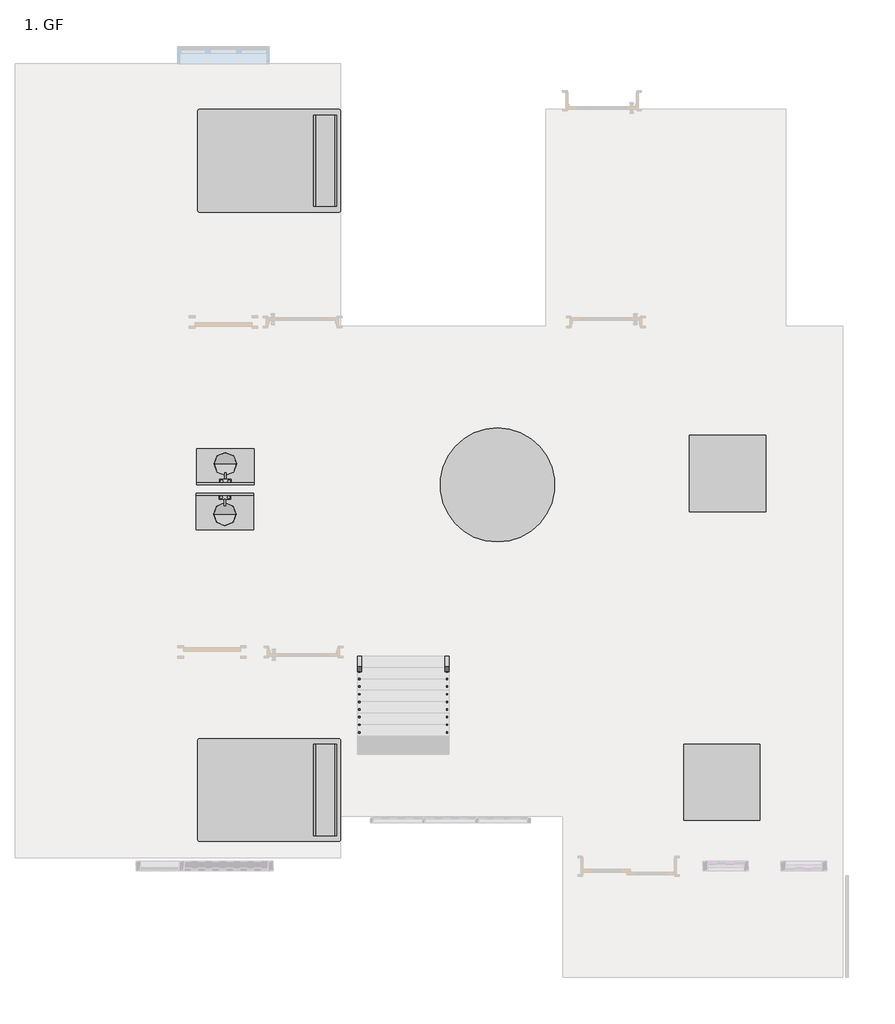
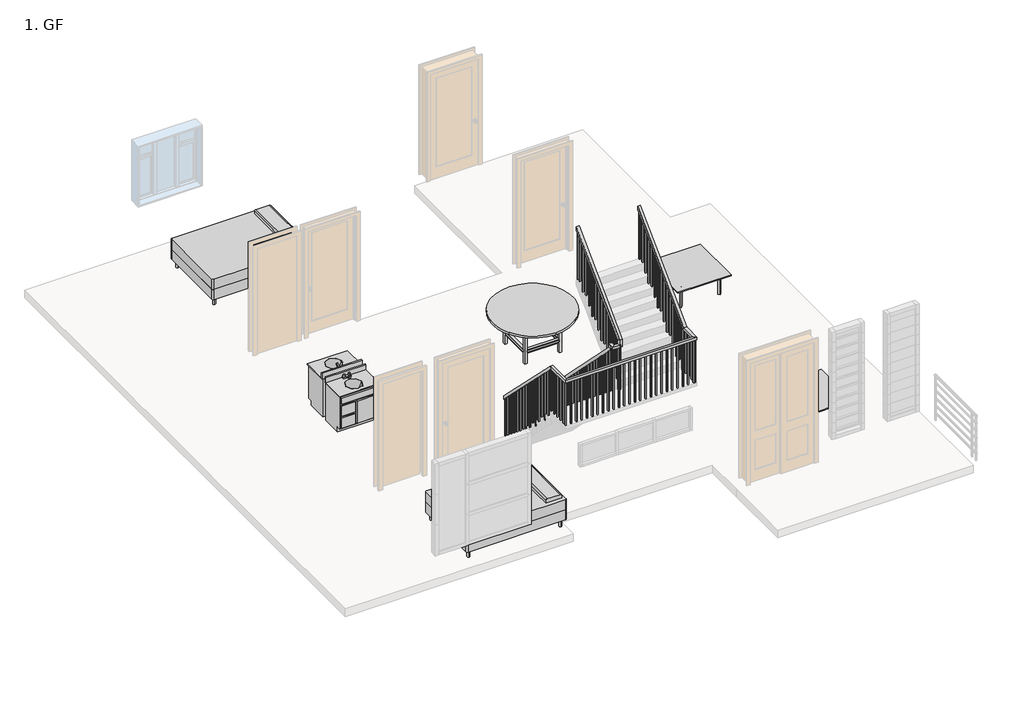
# One storey, part 3 of 3: 5 furniture elements, 2 flow terminals, 2 railings.
"""IFC4 building model written with IfcOpenShell, lengths in millimetres."""

from ifc_helpers import new_model, si_unit, frame, origin, place, context, project, spatial, polyline, outline, extrude, faceted_brep, transform, mapped, element, save
from components import flow_terminal_15267b2a, furniture_7b9c1204, furniture_52ef1662, furniture_86cdcdde

model = new_model("IFC4")

# Units and contexts
model_context = context("Model", 3, world=origin())
ifc_project = project(units=[si_unit("LENGTHUNIT", "METRE", prefix="MILLI")], contexts=[model_context])

# Site, building, storey
site = spatial("IfcSite", under=ifc_project)
building = spatial("IfcBuilding", under=site)
storey = spatial("IfcBuildingStorey", under=building, Name="1. GF", Elevation=609.6)

# Flow terminals
placement = place(None, origin())
flow_terminal_shape = flow_terminal_15267b2a(model_context)
element("IfcFlowTerminal", 1, ObjectType="Lavatory - Vanity : 30\"x18\" - Private", at=placement, inside=storey, context=model_context, shape_type="MappedRepresentation", body=[
    mapped(flow_terminal_shape, transform((-4529.7749552, 4478.4722789, 609.6), x_axis=(0.0, 1.0, 0.0), y_axis=(-1.0, 0.0, 0.0), z_axis=(0.0, 0.0, 1.0))),
])
element("IfcFlowTerminal", 2, ObjectType="Lavatory - Vanity : 30\"x18\" - Private", at=placement, inside=storey, context=model_context, shape_type="MappedRepresentation", body=[
    mapped(flow_terminal_shape, transform((-4536.1249552, 4365.7597789, 609.6), x_axis=(0.0, -1.0, 0.0), y_axis=(1.0, 0.0, 0.0), z_axis=(0.0, 0.0, 1.0))),
])

# Furniture
furniture_shape = furniture_7b9c1204(model_context)
element("IfcFurniture", 3, ObjectType="40\" x 40\"", at=placement, inside=storey, context=model_context, shape_type="MappedRepresentation", body=[
    mapped(furniture_shape, transform((2231.2053727, 4691.6266846, 609.6), x_axis=(1.0, 0.0, 0.0), y_axis=(0.0, 1.0, 0.0), z_axis=(0.0, 0.0, 1.0))),
])
element("IfcFurniture", 4, ObjectType="40\" x 40\"", at=placement, inside=storey, context=model_context, shape_type="MappedRepresentation", body=[
    mapped(furniture_shape, transform((2155.0053727, 570.4766846, 609.6), x_axis=(1.0, 0.0, 0.0), y_axis=(0.0, 1.0, 0.0), z_axis=(0.0, 0.0, 1.0))),
])
furniture_2_shape = furniture_52ef1662(model_context)
element("IfcFurniture", 5, ObjectType="Bed-Standard : Double 54\" x 75\"", at=placement, inside=storey, context=model_context, shape_type="MappedRepresentation", body=[
    mapped(furniture_2_shape, transform((-3899.9798732, 9075.1045534, 609.6), x_axis=(0.0, -1.0, 0.0), y_axis=(1.0, 0.0, 0.0), z_axis=(0.0, 0.0, 1.0))),
])
element("IfcFurniture", 6, ObjectType="Bed-Standard : Double 54\" x 75\"", at=placement, inside=storey, context=model_context, shape_type="MappedRepresentation", body=[
    mapped(furniture_2_shape, transform((-3899.9798732, 680.4045534, 609.6), x_axis=(0.0, -1.0, 0.0), y_axis=(1.0, 0.0, 0.0), z_axis=(0.0, 0.0, 1.0))),
])
furniture_3_shape = furniture_86cdcdde(model_context)
element("IfcFurniture", 7, ObjectType="Table-Dining Round w Chairs : 60\" Diameter", at=placement, inside=storey, context=model_context, shape_type="MappedRepresentation", body=[
    mapped(furniture_3_shape, transform((-1001.2569224, 4664.1447174, 609.6), x_axis=(1.0, 0.0, 0.0), y_axis=(0.0, 1.0, 0.0), z_axis=(0.0, 0.0, 1.0))),
])

# Railings
element("IfcRailing", 8, ObjectType="Handrail - Rectangular", at=placement, inside=storey, context=model_context, shape_type="SolidModel", body=[
    faceted_brep([(-2713.6749552, 2193.2660289, 1676.4), (-2713.6749552, 2193.2660289, 1604.557951), (-2764.4749552, 2193.2660289, 1604.557951), (-2764.4749552, 2193.2660289, 1676.4), (-2713.6749552, 669.2660289, 3200.4), (-2713.6749552, 648.2239799, 3149.6), (-2764.4749552, 648.2239799, 3149.6), (-2764.4749552, 669.2660289, 3200.4), (-2713.6749552, 224.7660289, 3200.4), (-2713.6749552, 224.7660289, 3149.6), (-2764.4749552, 173.9660289, 3149.6), (-2764.4749552, 173.9660289, 3200.4), (-300.6749552, 224.7660289, 3200.4), (-300.6749552, 224.7660289, 3149.6), (-249.8749552, 173.9660289, 3149.6), (-249.8749552, 173.9660289, 3200.4), (-300.6749552, 516.8660289, 3200.4), (-300.6749552, 537.9080778, 3149.6), (-249.8749552, 537.9080778, 3149.6), (-249.8749552, 516.8660289, 3200.4), (-300.6749552, 2040.8660289, 4724.4), (-249.8749552, 2040.8660289, 4724.4), (-249.8749552, 2040.8660289, 4652.557951), (-300.6749552, 2040.8660289, 4652.557951)], [[[0, 1, 2, 3]], [[1, 0, 4, 5]], [[2, 1, 5, 6]], [[3, 2, 6, 7]], [[0, 3, 7, 4]], [[5, 4, 8, 9]], [[6, 5, 9, 10]], [[7, 6, 10, 11]], [[4, 7, 11, 8]], [[9, 8, 12, 13]], [[10, 9, 13, 14]], [[11, 10, 14, 15]], [[8, 11, 15, 12]], [[13, 12, 16, 17]], [[14, 13, 17, 18]], [[15, 14, 18, 19]], [[12, 15, 19, 16]], [[20, 21, 22, 23]], [[17, 16, 20, 23]], [[18, 17, 23, 22]], [[19, 18, 22, 21]], [[16, 19, 21, 20]]]),
    extrude(outline(polyline([(2018.6410289, 4630.332951), (2037.6910289, 4649.382951), (2037.6910289, 3657.6), (2018.6410289, 3657.6), (2018.6410289, 4630.332951)])), frame((-284.7999552, 0.0, 0.0), z_axis=(1.0, 0.0, 0.0), x_axis=(0.0, 1.0, 0.0)), (0.0, 0.0, 1.0), 19.05),
    extrude(outline(polyline([(1917.0410289, 4528.732951), (1936.0910289, 4547.782951), (1936.0910289, 3657.6), (1917.0410289, 3657.6), (1917.0410289, 4528.732951)])), frame((-284.7999552, 0.0, 0.0), z_axis=(1.0, 0.0, 0.0), x_axis=(0.0, 1.0, 0.0)), (0.0, 0.0, 1.0), 19.05),
    extrude(outline(polyline([(1815.4410289, 4427.132951), (1834.4910289, 4446.182951), (1834.4910289, 3505.2), (1815.4410289, 3505.2), (1815.4410289, 4427.132951)])), frame((-284.7999552, 0.0, 0.0), z_axis=(1.0, 0.0, 0.0), x_axis=(0.0, 1.0, 0.0)), (0.0, 0.0, 1.0), 19.05),
    extrude(outline(polyline([(1713.8410289, 4325.532951), (1732.8910289, 4344.582951), (1732.8910289, 3352.8), (1713.8410289, 3352.8), (1713.8410289, 4325.532951)])), frame((-284.7999552, 0.0, 0.0), z_axis=(1.0, 0.0, 0.0), x_axis=(0.0, 1.0, 0.0)), (0.0, 0.0, 1.0), 19.05),
    extrude(outline(polyline([(1612.2410289, 4223.932951), (1631.2910289, 4242.982951), (1631.2910289, 3352.8), (1612.2410289, 3352.8), (1612.2410289, 4223.932951)])), frame((-284.7999552, 0.0, 0.0), z_axis=(1.0, 0.0, 0.0), x_axis=(0.0, 1.0, 0.0)), (0.0, 0.0, 1.0), 19.05),
    extrude(outline(polyline([(1510.6410289, 4122.332951), (1529.6910289, 4141.382951), (1529.6910289, 3200.4), (1510.6410289, 3200.4), (1510.6410289, 4122.332951)])), frame((-284.7999552, 0.0, 0.0), z_axis=(1.0, 0.0, 0.0), x_axis=(0.0, 1.0, 0.0)), (0.0, 0.0, 1.0), 19.05),
    extrude(outline(polyline([(1409.0410289, 4020.732951), (1428.0910289, 4039.782951), (1428.0910289, 3048.0), (1409.0410289, 3048.0), (1409.0410289, 4020.732951)])), frame((-284.7999552, 0.0, 0.0), z_axis=(1.0, 0.0, 0.0), x_axis=(0.0, 1.0, 0.0)), (0.0, 0.0, 1.0), 19.05),
    extrude(outline(polyline([(1307.4410289, 3919.132951), (1326.4910289, 3938.182951), (1326.4910289, 3048.0), (1307.4410289, 3048.0), (1307.4410289, 3919.132951)])), frame((-284.7999552, 0.0, 0.0), z_axis=(1.0, 0.0, 0.0), x_axis=(0.0, 1.0, 0.0)), (0.0, 0.0, 1.0), 19.05),
    extrude(outline(polyline([(1205.8410289, 3817.532951), (1224.8910289, 3836.582951), (1224.8910289, 2895.6), (1205.8410289, 2895.6), (1205.8410289, 3817.532951)])), frame((-284.7999552, 0.0, 0.0), z_axis=(1.0, 0.0, 0.0), x_axis=(0.0, 1.0, 0.0)), (0.0, 0.0, 1.0), 19.05),
    extrude(outline(polyline([(1104.2410289, 3715.932951), (1123.2910289, 3734.982951), (1123.2910289, 2743.2), (1104.2410289, 2743.2), (1104.2410289, 3715.932951)])), frame((-284.7999552, 0.0, 0.0), z_axis=(1.0, 0.0, 0.0), x_axis=(0.0, 1.0, 0.0)), (0.0, 0.0, 1.0), 19.05),
    extrude(outline(polyline([(1002.6410289, 3614.332951), (1021.6910289, 3633.382951), (1021.6910289, 2743.2), (1002.6410289, 2743.2), (1002.6410289, 3614.332951)])), frame((-284.7999552, 0.0, 0.0), z_axis=(1.0, 0.0, 0.0), x_axis=(0.0, 1.0, 0.0)), (0.0, 0.0, 1.0), 19.05),
    extrude(outline(polyline([(901.0410289, 3512.732951), (920.0910289, 3531.782951), (920.0910289, 2590.8), (901.0410289, 2590.8), (901.0410289, 3512.732951)])), frame((-284.7999552, 0.0, 0.0), z_axis=(1.0, 0.0, 0.0), x_axis=(0.0, 1.0, 0.0)), (0.0, 0.0, 1.0), 19.05),
    extrude(outline(polyline([(799.4410289, 3411.132951), (818.4910289, 3430.182951), (818.4910289, 2438.4), (799.4410289, 2438.4), (799.4410289, 3411.132951)])), frame((-284.7999552, 0.0, 0.0), z_axis=(1.0, 0.0, 0.0), x_axis=(0.0, 1.0, 0.0)), (0.0, 0.0, 1.0), 19.05),
    extrude(outline(polyline([(697.8410289, 3309.532951), (716.8910289, 3328.582951), (716.8910289, 2438.4), (697.8410289, 2438.4), (697.8410289, 3309.532951)])), frame((-284.7999552, 0.0, 0.0), z_axis=(1.0, 0.0, 0.0), x_axis=(0.0, 1.0, 0.0)), (0.0, 0.0, 1.0), 19.05),
    extrude(outline(polyline([(596.2410289, 3207.932951), (615.2910289, 3226.982951), (615.2910289, 2286.0), (596.2410289, 2286.0), (596.2410289, 3207.932951)])), frame((-284.7999552, 0.0, 0.0), z_axis=(1.0, 0.0, 0.0), x_axis=(0.0, 1.0, 0.0)), (0.0, 0.0, 1.0), 19.05),
    extrude(outline(polyline([(-265.7499552, 494.6410289), (-284.7999552, 494.6410289), (-284.7999552, 513.6910289), (-265.7499552, 513.6910289), (-265.7499552, 494.6410289)])), frame((0.0, 0.0, 2286.0), z_axis=(0.0, 0.0, 1.0), x_axis=(1.0, 0.0, 0.0)), (0.0, 0.0, 1.0), 863.6),
    extrude(outline(polyline([(-265.7499552, 393.0410289), (-284.7999552, 393.0410289), (-284.7999552, 412.0910289), (-265.7499552, 412.0910289), (-265.7499552, 393.0410289)])), frame((0.0, 0.0, 2286.0), z_axis=(0.0, 0.0, 1.0), x_axis=(1.0, 0.0, 0.0)), (0.0, 0.0, 1.0), 863.6),
    extrude(outline(polyline([(-265.7499552, 291.4410289), (-284.7999552, 291.4410289), (-284.7999552, 310.4910289), (-265.7499552, 310.4910289), (-265.7499552, 291.4410289)])), frame((0.0, 0.0, 2286.0), z_axis=(0.0, 0.0, 1.0), x_axis=(1.0, 0.0, 0.0)), (0.0, 0.0, 1.0), 863.6),
    extrude(outline(polyline([(-310.1999552, 189.8410289), (-310.1999552, 208.8910289), (-291.1499552, 208.8910289), (-291.1499552, 189.8410289), (-310.1999552, 189.8410289)])), frame((0.0, 0.0, 2286.0), z_axis=(0.0, 0.0, 1.0), x_axis=(1.0, 0.0, 0.0)), (0.0, 0.0, 1.0), 863.6),
    extrude(outline(polyline([(-411.7999552, 189.8410289), (-411.7999552, 208.8910289), (-392.7499552, 208.8910289), (-392.7499552, 189.8410289), (-411.7999552, 189.8410289)])), frame((0.0, 0.0, 2286.0), z_axis=(0.0, 0.0, 1.0), x_axis=(1.0, 0.0, 0.0)), (0.0, 0.0, 1.0), 863.6),
    extrude(outline(polyline([(-513.3999552, 189.8410289), (-513.3999552, 208.8910289), (-494.3499552, 208.8910289), (-494.3499552, 189.8410289), (-513.3999552, 189.8410289)])), frame((0.0, 0.0, 2286.0), z_axis=(0.0, 0.0, 1.0), x_axis=(1.0, 0.0, 0.0)), (0.0, 0.0, 1.0), 863.6),
    extrude(outline(polyline([(-614.9999552, 189.8410289), (-614.9999552, 208.8910289), (-595.9499552, 208.8910289), (-595.9499552, 189.8410289), (-614.9999552, 189.8410289)])), frame((0.0, 0.0, 2286.0), z_axis=(0.0, 0.0, 1.0), x_axis=(1.0, 0.0, 0.0)), (0.0, 0.0, 1.0), 863.6),
    extrude(outline(polyline([(-716.5999552, 189.8410289), (-716.5999552, 208.8910289), (-697.5499552, 208.8910289), (-697.5499552, 189.8410289), (-716.5999552, 189.8410289)])), frame((0.0, 0.0, 2286.0), z_axis=(0.0, 0.0, 1.0), x_axis=(1.0, 0.0, 0.0)), (0.0, 0.0, 1.0), 863.6),
    extrude(outline(polyline([(-818.1999552, 189.8410289), (-818.1999552, 208.8910289), (-799.1499552, 208.8910289), (-799.1499552, 189.8410289), (-818.1999552, 189.8410289)])), frame((0.0, 0.0, 2286.0), z_axis=(0.0, 0.0, 1.0), x_axis=(1.0, 0.0, 0.0)), (0.0, 0.0, 1.0), 863.6),
    extrude(outline(polyline([(-919.7999552, 189.8410289), (-919.7999552, 208.8910289), (-900.7499552, 208.8910289), (-900.7499552, 189.8410289), (-919.7999552, 189.8410289)])), frame((0.0, 0.0, 2286.0), z_axis=(0.0, 0.0, 1.0), x_axis=(1.0, 0.0, 0.0)), (0.0, 0.0, 1.0), 863.6),
    extrude(outline(polyline([(-1021.3999552, 189.8410289), (-1021.3999552, 208.8910289), (-1002.3499552, 208.8910289), (-1002.3499552, 189.8410289), (-1021.3999552, 189.8410289)])), frame((0.0, 0.0, 2286.0), z_axis=(0.0, 0.0, 1.0), x_axis=(1.0, 0.0, 0.0)), (0.0, 0.0, 1.0), 863.6),
    extrude(outline(polyline([(-1122.9999552, 189.8410289), (-1122.9999552, 208.8910289), (-1103.9499552, 208.8910289), (-1103.9499552, 189.8410289), (-1122.9999552, 189.8410289)])), frame((0.0, 0.0, 2286.0), z_axis=(0.0, 0.0, 1.0), x_axis=(1.0, 0.0, 0.0)), (0.0, 0.0, 1.0), 863.6),
    extrude(outline(polyline([(-1224.5999552, 189.8410289), (-1224.5999552, 208.8910289), (-1205.5499552, 208.8910289), (-1205.5499552, 189.8410289), (-1224.5999552, 189.8410289)])), frame((0.0, 0.0, 2286.0), z_axis=(0.0, 0.0, 1.0), x_axis=(1.0, 0.0, 0.0)), (0.0, 0.0, 1.0), 863.6),
    extrude(outline(polyline([(-1326.1999552, 189.8410289), (-1326.1999552, 208.8910289), (-1307.1499552, 208.8910289), (-1307.1499552, 189.8410289), (-1326.1999552, 189.8410289)])), frame((0.0, 0.0, 2286.0), z_axis=(0.0, 0.0, 1.0), x_axis=(1.0, 0.0, 0.0)), (0.0, 0.0, 1.0), 863.6),
    extrude(outline(polyline([(-1427.7999552, 189.8410289), (-1427.7999552, 208.8910289), (-1408.7499552, 208.8910289), (-1408.7499552, 189.8410289), (-1427.7999552, 189.8410289)])), frame((0.0, 0.0, 2286.0), z_axis=(0.0, 0.0, 1.0), x_axis=(1.0, 0.0, 0.0)), (0.0, 0.0, 1.0), 863.6),
    extrude(outline(polyline([(-1529.3999552, 189.8410289), (-1529.3999552, 208.8910289), (-1510.3499552, 208.8910289), (-1510.3499552, 189.8410289), (-1529.3999552, 189.8410289)])), frame((0.0, 0.0, 2286.0), z_axis=(0.0, 0.0, 1.0), x_axis=(1.0, 0.0, 0.0)), (0.0, 0.0, 1.0), 863.6),
    extrude(outline(polyline([(-1630.9999552, 189.8410289), (-1630.9999552, 208.8910289), (-1611.9499552, 208.8910289), (-1611.9499552, 189.8410289), (-1630.9999552, 189.8410289)])), frame((0.0, 0.0, 2286.0), z_axis=(0.0, 0.0, 1.0), x_axis=(1.0, 0.0, 0.0)), (0.0, 0.0, 1.0), 863.6),
    extrude(outline(polyline([(-1732.5999552, 189.8410289), (-1732.5999552, 208.8910289), (-1713.5499552, 208.8910289), (-1713.5499552, 189.8410289), (-1732.5999552, 189.8410289)])), frame((0.0, 0.0, 2286.0), z_axis=(0.0, 0.0, 1.0), x_axis=(1.0, 0.0, 0.0)), (0.0, 0.0, 1.0), 863.6),
    extrude(outline(polyline([(-1834.1999552, 189.8410289), (-1834.1999552, 208.8910289), (-1815.1499552, 208.8910289), (-1815.1499552, 189.8410289), (-1834.1999552, 189.8410289)])), frame((0.0, 0.0, 2286.0), z_axis=(0.0, 0.0, 1.0), x_axis=(1.0, 0.0, 0.0)), (0.0, 0.0, 1.0), 863.6),
    extrude(outline(polyline([(-1935.7999552, 189.8410289), (-1935.7999552, 208.8910289), (-1916.7499552, 208.8910289), (-1916.7499552, 189.8410289), (-1935.7999552, 189.8410289)])), frame((0.0, 0.0, 2286.0), z_axis=(0.0, 0.0, 1.0), x_axis=(1.0, 0.0, 0.0)), (0.0, 0.0, 1.0), 863.6),
    extrude(outline(polyline([(-2037.3999552, 189.8410289), (-2037.3999552, 208.8910289), (-2018.3499552, 208.8910289), (-2018.3499552, 189.8410289), (-2037.3999552, 189.8410289)])), frame((0.0, 0.0, 2286.0), z_axis=(0.0, 0.0, 1.0), x_axis=(1.0, 0.0, 0.0)), (0.0, 0.0, 1.0), 863.6),
    extrude(outline(polyline([(-2138.9999552, 189.8410289), (-2138.9999552, 208.8910289), (-2119.9499552, 208.8910289), (-2119.9499552, 189.8410289), (-2138.9999552, 189.8410289)])), frame((0.0, 0.0, 2286.0), z_axis=(0.0, 0.0, 1.0), x_axis=(1.0, 0.0, 0.0)), (0.0, 0.0, 1.0), 863.6),
    extrude(outline(polyline([(-2240.5999552, 189.8410289), (-2240.5999552, 208.8910289), (-2221.5499552, 208.8910289), (-2221.5499552, 189.8410289), (-2240.5999552, 189.8410289)])), frame((0.0, 0.0, 2286.0), z_axis=(0.0, 0.0, 1.0), x_axis=(1.0, 0.0, 0.0)), (0.0, 0.0, 1.0), 863.6),
    extrude(outline(polyline([(-2342.1999552, 189.8410289), (-2342.1999552, 208.8910289), (-2323.1499552, 208.8910289), (-2323.1499552, 189.8410289), (-2342.1999552, 189.8410289)])), frame((0.0, 0.0, 2286.0), z_axis=(0.0, 0.0, 1.0), x_axis=(1.0, 0.0, 0.0)), (0.0, 0.0, 1.0), 863.6),
    extrude(outline(polyline([(-2443.7999552, 189.8410289), (-2443.7999552, 208.8910289), (-2424.7499552, 208.8910289), (-2424.7499552, 189.8410289), (-2443.7999552, 189.8410289)])), frame((0.0, 0.0, 2286.0), z_axis=(0.0, 0.0, 1.0), x_axis=(1.0, 0.0, 0.0)), (0.0, 0.0, 1.0), 863.6),
    extrude(outline(polyline([(-2545.3999552, 189.8410289), (-2545.3999552, 208.8910289), (-2526.3499552, 208.8910289), (-2526.3499552, 189.8410289), (-2545.3999552, 189.8410289)])), frame((0.0, 0.0, 2286.0), z_axis=(0.0, 0.0, 1.0), x_axis=(1.0, 0.0, 0.0)), (0.0, 0.0, 1.0), 863.6),
    extrude(outline(polyline([(-2646.9999552, 189.8410289), (-2646.9999552, 208.8910289), (-2627.9499552, 208.8910289), (-2627.9499552, 189.8410289), (-2646.9999552, 189.8410289)])), frame((0.0, 0.0, 2286.0), z_axis=(0.0, 0.0, 1.0), x_axis=(1.0, 0.0, 0.0)), (0.0, 0.0, 1.0), 863.6),
    extrude(outline(polyline([(-2748.5999552, 272.3910289), (-2729.5499552, 272.3910289), (-2729.5499552, 253.3410289), (-2748.5999552, 253.3410289), (-2748.5999552, 272.3910289)])), frame((0.0, 0.0, 2286.0), z_axis=(0.0, 0.0, 1.0), x_axis=(1.0, 0.0, 0.0)), (0.0, 0.0, 1.0), 863.6),
    extrude(outline(polyline([(-2748.5999552, 373.9910289), (-2729.5499552, 373.9910289), (-2729.5499552, 354.9410289), (-2748.5999552, 354.9410289), (-2748.5999552, 373.9910289)])), frame((0.0, 0.0, 2286.0), z_axis=(0.0, 0.0, 1.0), x_axis=(1.0, 0.0, 0.0)), (0.0, 0.0, 1.0), 863.6),
    extrude(outline(polyline([(-2748.5999552, 475.5910289), (-2729.5499552, 475.5910289), (-2729.5499552, 456.5410289), (-2748.5999552, 456.5410289), (-2748.5999552, 475.5910289)])), frame((0.0, 0.0, 2286.0), z_axis=(0.0, 0.0, 1.0), x_axis=(1.0, 0.0, 0.0)), (0.0, 0.0, 1.0), 863.6),
    extrude(outline(polyline([(-2748.5999552, 577.1910289), (-2729.5499552, 577.1910289), (-2729.5499552, 558.1410289), (-2748.5999552, 558.1410289), (-2748.5999552, 577.1910289)])), frame((0.0, 0.0, 2286.0), z_axis=(0.0, 0.0, 1.0), x_axis=(1.0, 0.0, 0.0)), (0.0, 0.0, 1.0), 863.6),
    extrude(outline(polyline([(659.7410289, 3138.082951), (678.7910289, 3119.032951), (678.7910289, 2286.0), (659.7410289, 2286.0), (659.7410289, 3138.082951)])), frame((-2748.5999552, 0.0, 0.0), z_axis=(1.0, 0.0, 0.0), x_axis=(0.0, 1.0, 0.0)), (0.0, 0.0, 1.0), 19.05),
    extrude(outline(polyline([(761.3410289, 3036.482951), (780.3910289, 3017.432951), (780.3910289, 2133.6), (761.3410289, 2133.6), (761.3410289, 3036.482951)])), frame((-2748.5999552, 0.0, 0.0), z_axis=(1.0, 0.0, 0.0), x_axis=(0.0, 1.0, 0.0)), (0.0, 0.0, 1.0), 19.05),
    extrude(outline(polyline([(862.9410289, 2934.882951), (881.9910289, 2915.832951), (881.9910289, 1981.2), (862.9410289, 1981.2), (862.9410289, 2934.882951)])), frame((-2748.5999552, 0.0, 0.0), z_axis=(1.0, 0.0, 0.0), x_axis=(0.0, 1.0, 0.0)), (0.0, 0.0, 1.0), 19.05),
    extrude(outline(polyline([(964.5410289, 2833.282951), (983.5910289, 2814.232951), (983.5910289, 1981.2), (964.5410289, 1981.2), (964.5410289, 2833.282951)])), frame((-2748.5999552, 0.0, 0.0), z_axis=(1.0, 0.0, 0.0), x_axis=(0.0, 1.0, 0.0)), (0.0, 0.0, 1.0), 19.05),
    extrude(outline(polyline([(1066.1410289, 2731.682951), (1085.1910289, 2712.632951), (1085.1910289, 1828.8), (1066.1410289, 1828.8), (1066.1410289, 2731.682951)])), frame((-2748.5999552, 0.0, 0.0), z_axis=(1.0, 0.0, 0.0), x_axis=(0.0, 1.0, 0.0)), (0.0, 0.0, 1.0), 19.05),
    extrude(outline(polyline([(1167.7410289, 2630.082951), (1186.7910289, 2611.032951), (1186.7910289, 1676.4), (1167.7410289, 1676.4), (1167.7410289, 2630.082951)])), frame((-2748.5999552, 0.0, 0.0), z_axis=(1.0, 0.0, 0.0), x_axis=(0.0, 1.0, 0.0)), (0.0, 0.0, 1.0), 19.05),
    extrude(outline(polyline([(1269.3410289, 2528.482951), (1288.3910289, 2509.432951), (1288.3910289, 1676.4), (1269.3410289, 1676.4), (1269.3410289, 2528.482951)])), frame((-2748.5999552, 0.0, 0.0), z_axis=(1.0, 0.0, 0.0), x_axis=(0.0, 1.0, 0.0)), (0.0, 0.0, 1.0), 19.05),
    extrude(outline(polyline([(1370.9410289, 2426.882951), (1389.9910289, 2407.832951), (1389.9910289, 1524.0), (1370.9410289, 1524.0), (1370.9410289, 2426.882951)])), frame((-2748.5999552, 0.0, 0.0), z_axis=(1.0, 0.0, 0.0), x_axis=(0.0, 1.0, 0.0)), (0.0, 0.0, 1.0), 19.05),
    extrude(outline(polyline([(1472.5410289, 2325.282951), (1491.5910289, 2306.232951), (1491.5910289, 1371.6), (1472.5410289, 1371.6), (1472.5410289, 2325.282951)])), frame((-2748.5999552, 0.0, 0.0), z_axis=(1.0, 0.0, 0.0), x_axis=(0.0, 1.0, 0.0)), (0.0, 0.0, 1.0), 19.05),
    extrude(outline(polyline([(1574.1410289, 2223.682951), (1593.1910289, 2204.632951), (1593.1910289, 1371.6), (1574.1410289, 1371.6), (1574.1410289, 2223.682951)])), frame((-2748.5999552, 0.0, 0.0), z_axis=(1.0, 0.0, 0.0), x_axis=(0.0, 1.0, 0.0)), (0.0, 0.0, 1.0), 19.05),
    extrude(outline(polyline([(1675.7410289, 2122.082951), (1694.7910289, 2103.032951), (1694.7910289, 1219.2), (1675.7410289, 1219.2), (1675.7410289, 2122.082951)])), frame((-2748.5999552, 0.0, 0.0), z_axis=(1.0, 0.0, 0.0), x_axis=(0.0, 1.0, 0.0)), (0.0, 0.0, 1.0), 19.05),
    extrude(outline(polyline([(1777.3410289, 2020.482951), (1796.3910289, 2001.432951), (1796.3910289, 1066.8), (1777.3410289, 1066.8), (1777.3410289, 2020.482951)])), frame((-2748.5999552, 0.0, 0.0), z_axis=(1.0, 0.0, 0.0), x_axis=(0.0, 1.0, 0.0)), (0.0, 0.0, 1.0), 19.05),
    extrude(outline(polyline([(1878.9410289, 1918.882951), (1897.9910289, 1899.832951), (1897.9910289, 1066.8), (1878.9410289, 1066.8), (1878.9410289, 1918.882951)])), frame((-2748.5999552, 0.0, 0.0), z_axis=(1.0, 0.0, 0.0), x_axis=(0.0, 1.0, 0.0)), (0.0, 0.0, 1.0), 19.05),
    extrude(outline(polyline([(1980.5410289, 1817.282951), (1999.5910289, 1798.232951), (1999.5910289, 914.4), (1980.5410289, 914.4), (1980.5410289, 1817.282951)])), frame((-2748.5999552, 0.0, 0.0), z_axis=(1.0, 0.0, 0.0), x_axis=(0.0, 1.0, 0.0)), (0.0, 0.0, 1.0), 19.05),
    extrude(outline(polyline([(2082.1410289, 1715.682951), (2101.1910289, 1696.632951), (2101.1910289, 762.0), (2082.1410289, 762.0), (2082.1410289, 1715.682951)])), frame((-2748.5999552, 0.0, 0.0), z_axis=(1.0, 0.0, 0.0), x_axis=(0.0, 1.0, 0.0)), (0.0, 0.0, 1.0), 19.05),
    extrude(outline(polyline([(-284.7999552, 189.8410289), (-284.7999552, 208.8910289), (-265.7499552, 208.8910289), (-265.7499552, 189.8410289), (-284.7999552, 189.8410289)])), frame((0.0, 0.0, 2286.0), z_axis=(0.0, 0.0, 1.0), x_axis=(1.0, 0.0, 0.0)), (0.0, 0.0, 1.0), 863.6),
    extrude(outline(polyline([(-2748.5999552, 208.8910289), (-2729.5499552, 208.8910289), (-2729.5499552, 189.8410289), (-2748.5999552, 189.8410289), (-2748.5999552, 208.8910289)])), frame((0.0, 0.0, 2286.0), z_axis=(0.0, 0.0, 1.0), x_axis=(1.0, 0.0, 0.0)), (0.0, 0.0, 1.0), 863.6),
    extrude(outline(polyline([(2021.8160289, 4633.507951), (2040.8660289, 4652.557951), (2040.8660289, 3657.6), (2021.8160289, 3657.6), (2021.8160289, 4633.507951)])), frame((-284.7999552, 0.0, 0.0), z_axis=(1.0, 0.0, 0.0), x_axis=(0.0, 1.0, 0.0)), (0.0, 0.0, 1.0), 19.05),
    extrude(outline(polyline([(2174.2160289, 1623.607951), (2193.2660289, 1604.557951), (2193.2660289, 762.0), (2174.2160289, 762.0), (2174.2160289, 1623.607951)])), frame((-2748.5999552, 0.0, 0.0), z_axis=(1.0, 0.0, 0.0), x_axis=(0.0, 1.0, 0.0)), (0.0, 0.0, 1.0), 19.05),
])
element("IfcRailing", 9, ObjectType="Handrail - Rectangular", at=placement, inside=storey, context=model_context, shape_type="SolidModel", body=[
    faceted_brep([(-1545.2749552, 2193.2660289, 1676.4), (-1545.2749552, 2193.2660289, 1604.557951), (-1596.0749552, 2193.2660289, 1604.557951), (-1596.0749552, 2193.2660289, 1676.4), (-1545.2749552, 745.4660289, 3124.2), (-1545.2749552, 694.6660289, 3103.157951), (-1596.0749552, 694.6660289, 3103.157951), (-1596.0749552, 745.4660289, 3124.2), (-1545.2749552, 745.4660289, 3200.4), (-1545.2749552, 694.6660289, 3149.6), (-1596.0749552, 694.6660289, 3149.6), (-1596.0749552, 745.4660289, 3200.4), (-1545.2749552, 669.2660289, 3200.4), (-1545.2749552, 669.2660289, 3149.6), (-1596.0749552, 618.4660289, 3149.6), (-1596.0749552, 618.4660289, 3200.4), (-1469.0749552, 669.2660289, 3200.4), (-1469.0749552, 669.2660289, 3149.6), (-1469.0749552, 618.4660289, 3149.6), (-1469.0749552, 618.4660289, 3200.4), (-1443.6749552, 669.2660289, 3200.4), (-1443.6749552, 618.4660289, 3200.4), (-1443.6749552, 618.4660289, 3149.6), (-1443.6749552, 669.2660289, 3149.6)], [[[0, 1, 2, 3]], [[1, 0, 4, 5]], [[2, 1, 5, 6]], [[3, 2, 6, 7]], [[0, 3, 7, 4]], [[5, 4, 8, 9]], [[6, 5, 9, 10]], [[7, 6, 10, 11]], [[4, 7, 11, 8]], [[9, 8, 12, 13]], [[10, 9, 13, 14]], [[11, 10, 14, 15]], [[8, 11, 15, 12]], [[13, 12, 16, 17]], [[14, 13, 17, 18]], [[15, 14, 18, 19]], [[12, 15, 19, 16]], [[20, 21, 22, 23]], [[17, 16, 20, 23]], [[18, 17, 23, 22]], [[19, 18, 22, 21]], [[16, 19, 21, 20]]]),
    faceted_brep([(-1469.0749552, 669.2660289, 3200.4), (-1418.2749552, 669.2660289, 3149.6), (-1418.2749552, 618.4660289, 3149.6), (-1469.0749552, 618.4660289, 3200.4), (-1469.0749552, 669.2660289, 3280.957951), (-1469.0749552, 618.4660289, 3302.0), (-1418.2749552, 618.4660289, 3302.0), (-1418.2749552, 669.2660289, 3280.957951)], [[[0, 1, 2, 3]], [[4, 5, 6, 7]], [[1, 0, 4, 7]], [[2, 1, 7, 6]], [[3, 2, 6, 5]], [[0, 3, 5, 4]]]),
    faceted_brep([(-1469.0749552, 618.4660289, 3302.0), (-1469.0749552, 669.2660289, 3280.957951), (-1418.2749552, 669.2660289, 3280.957951), (-1418.2749552, 618.4660289, 3302.0), (-1469.0749552, 2040.8660289, 4724.4), (-1418.2749552, 2040.8660289, 4724.4), (-1418.2749552, 2040.8660289, 4652.557951), (-1469.0749552, 2040.8660289, 4652.557951)], [[[0, 1, 2, 3]], [[4, 5, 6, 7]], [[1, 0, 4, 7]], [[2, 1, 7, 6]], [[3, 2, 6, 5]], [[0, 3, 5, 4]]]),
    extrude(outline(polyline([(1974.1910289, 4585.882951), (1974.1910289, 3657.6), (1955.1410289, 3657.6), (1955.1410289, 4566.832951), (1974.1910289, 4585.882951)])), frame((-1453.1999552, 0.0, 0.0), z_axis=(1.0, 0.0, 0.0), x_axis=(0.0, 1.0, 0.0)), (0.0, 0.0, 1.0), 19.05),
    extrude(outline(polyline([(1872.5910289, 4484.282951), (1872.5910289, 3505.2), (1853.5410289, 3505.2), (1853.5410289, 4465.232951), (1872.5910289, 4484.282951)])), frame((-1453.1999552, 0.0, 0.0), z_axis=(1.0, 0.0, 0.0), x_axis=(0.0, 1.0, 0.0)), (0.0, 0.0, 1.0), 19.05),
    extrude(outline(polyline([(1770.9910289, 4382.682951), (1770.9910289, 3505.2), (1751.9410289, 3505.2), (1751.9410289, 4363.632951), (1770.9910289, 4382.682951)])), frame((-1453.1999552, 0.0, 0.0), z_axis=(1.0, 0.0, 0.0), x_axis=(0.0, 1.0, 0.0)), (0.0, 0.0, 1.0), 19.05),
    extrude(outline(polyline([(1669.3910289, 4281.082951), (1669.3910289, 3352.8), (1650.3410289, 3352.8), (1650.3410289, 4262.032951), (1669.3910289, 4281.082951)])), frame((-1453.1999552, 0.0, 0.0), z_axis=(1.0, 0.0, 0.0), x_axis=(0.0, 1.0, 0.0)), (0.0, 0.0, 1.0), 19.05),
    extrude(outline(polyline([(1567.7910289, 4179.482951), (1567.7910289, 3200.4), (1548.7410289, 3200.4), (1548.7410289, 4160.432951), (1567.7910289, 4179.482951)])), frame((-1453.1999552, 0.0, 0.0), z_axis=(1.0, 0.0, 0.0), x_axis=(0.0, 1.0, 0.0)), (0.0, 0.0, 1.0), 19.05),
    extrude(outline(polyline([(1466.1910289, 4077.882951), (1466.1910289, 3200.4), (1447.1410289, 3200.4), (1447.1410289, 4058.832951), (1466.1910289, 4077.882951)])), frame((-1453.1999552, 0.0, 0.0), z_axis=(1.0, 0.0, 0.0), x_axis=(0.0, 1.0, 0.0)), (0.0, 0.0, 1.0), 19.05),
    extrude(outline(polyline([(1364.5910289, 3976.282951), (1364.5910289, 3048.0), (1345.5410289, 3048.0), (1345.5410289, 3957.232951), (1364.5910289, 3976.282951)])), frame((-1453.1999552, 0.0, 0.0), z_axis=(1.0, 0.0, 0.0), x_axis=(0.0, 1.0, 0.0)), (0.0, 0.0, 1.0), 19.05),
    extrude(outline(polyline([(1262.9910289, 3874.682951), (1262.9910289, 2895.6), (1243.9410289, 2895.6), (1243.9410289, 3855.632951), (1262.9910289, 3874.682951)])), frame((-1453.1999552, 0.0, 0.0), z_axis=(1.0, 0.0, 0.0), x_axis=(0.0, 1.0, 0.0)), (0.0, 0.0, 1.0), 19.05),
    extrude(outline(polyline([(1161.3910289, 3773.082951), (1161.3910289, 2895.6), (1142.3410289, 2895.6), (1142.3410289, 3754.032951), (1161.3910289, 3773.082951)])), frame((-1453.1999552, 0.0, 0.0), z_axis=(1.0, 0.0, 0.0), x_axis=(0.0, 1.0, 0.0)), (0.0, 0.0, 1.0), 19.05),
    extrude(outline(polyline([(1059.7910289, 3671.482951), (1059.7910289, 2743.2), (1040.7410289, 2743.2), (1040.7410289, 3652.432951), (1059.7910289, 3671.482951)])), frame((-1453.1999552, 0.0, 0.0), z_axis=(1.0, 0.0, 0.0), x_axis=(0.0, 1.0, 0.0)), (0.0, 0.0, 1.0), 19.05),
    extrude(outline(polyline([(958.1910289, 3569.882951), (958.1910289, 2590.8), (939.1410289, 2590.8), (939.1410289, 3550.832951), (958.1910289, 3569.882951)])), frame((-1453.1999552, 0.0, 0.0), z_axis=(1.0, 0.0, 0.0), x_axis=(0.0, 1.0, 0.0)), (0.0, 0.0, 1.0), 19.05),
    extrude(outline(polyline([(856.5910289, 3468.282951), (856.5910289, 2590.8), (837.5410289, 2590.8), (837.5410289, 3449.232951), (856.5910289, 3468.282951)])), frame((-1453.1999552, 0.0, 0.0), z_axis=(1.0, 0.0, 0.0), x_axis=(0.0, 1.0, 0.0)), (0.0, 0.0, 1.0), 19.05),
    extrude(outline(polyline([(754.9910289, 3366.682951), (754.9910289, 2438.4), (735.9410289, 2438.4), (735.9410289, 3347.632951), (754.9910289, 3366.682951)])), frame((-1453.1999552, 0.0, 0.0), z_axis=(1.0, 0.0, 0.0), x_axis=(0.0, 1.0, 0.0)), (0.0, 0.0, 1.0), 19.05),
    extrude(outline(polyline([(-1478.5999552, 653.3910289), (-1459.5499552, 653.3910289), (-1459.5499552, 634.3410289), (-1478.5999552, 634.3410289), (-1478.5999552, 653.3910289)])), frame((0.0, 0.0, 2286.0), z_axis=(0.0, 0.0, 1.0), x_axis=(1.0, 0.0, 0.0)), (0.0, 0.0, 1.0), 863.6),
    extrude(outline(polyline([(-1561.1499552, 678.7910289), (-1561.1499552, 659.7410289), (-1580.1999552, 659.7410289), (-1580.1999552, 678.7910289), (-1561.1499552, 678.7910289)])), frame((0.0, 0.0, 2286.0), z_axis=(0.0, 0.0, 1.0), x_axis=(1.0, 0.0, 0.0)), (0.0, 0.0, 1.0), 863.6),
    extrude(outline(polyline([(780.3910289, 3017.432951), (780.3910289, 2133.6), (761.3410289, 2133.6), (761.3410289, 3036.482951), (780.3910289, 3017.432951)])), frame((-1580.1999552, 0.0, 0.0), z_axis=(1.0, 0.0, 0.0), x_axis=(0.0, 1.0, 0.0)), (0.0, 0.0, 1.0), 19.05),
    extrude(outline(polyline([(881.9910289, 2915.832951), (881.9910289, 1981.2), (862.9410289, 1981.2), (862.9410289, 2934.882951), (881.9910289, 2915.832951)])), frame((-1580.1999552, 0.0, 0.0), z_axis=(1.0, 0.0, 0.0), x_axis=(0.0, 1.0, 0.0)), (0.0, 0.0, 1.0), 19.05),
    extrude(outline(polyline([(983.5910289, 2814.232951), (983.5910289, 1981.2), (964.5410289, 1981.2), (964.5410289, 2833.282951), (983.5910289, 2814.232951)])), frame((-1580.1999552, 0.0, 0.0), z_axis=(1.0, 0.0, 0.0), x_axis=(0.0, 1.0, 0.0)), (0.0, 0.0, 1.0), 19.05),
    extrude(outline(polyline([(1085.1910289, 2712.632951), (1085.1910289, 1828.8), (1066.1410289, 1828.8), (1066.1410289, 2731.682951), (1085.1910289, 2712.632951)])), frame((-1580.1999552, 0.0, 0.0), z_axis=(1.0, 0.0, 0.0), x_axis=(0.0, 1.0, 0.0)), (0.0, 0.0, 1.0), 19.05),
    extrude(outline(polyline([(1186.7910289, 2611.032951), (1186.7910289, 1676.4), (1167.7410289, 1676.4), (1167.7410289, 2630.082951), (1186.7910289, 2611.032951)])), frame((-1580.1999552, 0.0, 0.0), z_axis=(1.0, 0.0, 0.0), x_axis=(0.0, 1.0, 0.0)), (0.0, 0.0, 1.0), 19.05),
    extrude(outline(polyline([(1288.3910289, 2509.432951), (1288.3910289, 1676.4), (1269.3410289, 1676.4), (1269.3410289, 2528.482951), (1288.3910289, 2509.432951)])), frame((-1580.1999552, 0.0, 0.0), z_axis=(1.0, 0.0, 0.0), x_axis=(0.0, 1.0, 0.0)), (0.0, 0.0, 1.0), 19.05),
    extrude(outline(polyline([(1389.9910289, 2407.832951), (1389.9910289, 1524.0), (1370.9410289, 1524.0), (1370.9410289, 2426.882951), (1389.9910289, 2407.832951)])), frame((-1580.1999552, 0.0, 0.0), z_axis=(1.0, 0.0, 0.0), x_axis=(0.0, 1.0, 0.0)), (0.0, 0.0, 1.0), 19.05),
    extrude(outline(polyline([(1491.5910289, 2306.232951), (1491.5910289, 1371.6), (1472.5410289, 1371.6), (1472.5410289, 2325.282951), (1491.5910289, 2306.232951)])), frame((-1580.1999552, 0.0, 0.0), z_axis=(1.0, 0.0, 0.0), x_axis=(0.0, 1.0, 0.0)), (0.0, 0.0, 1.0), 19.05),
    extrude(outline(polyline([(1593.1910289, 2204.632951), (1593.1910289, 1371.6), (1574.1410289, 1371.6), (1574.1410289, 2223.682951), (1593.1910289, 2204.632951)])), frame((-1580.1999552, 0.0, 0.0), z_axis=(1.0, 0.0, 0.0), x_axis=(0.0, 1.0, 0.0)), (0.0, 0.0, 1.0), 19.05),
    extrude(outline(polyline([(1694.7910289, 2103.032951), (1694.7910289, 1219.2), (1675.7410289, 1219.2), (1675.7410289, 2122.082951), (1694.7910289, 2103.032951)])), frame((-1580.1999552, 0.0, 0.0), z_axis=(1.0, 0.0, 0.0), x_axis=(0.0, 1.0, 0.0)), (0.0, 0.0, 1.0), 19.05),
    extrude(outline(polyline([(1796.3910289, 2001.432951), (1796.3910289, 1066.8), (1777.3410289, 1066.8), (1777.3410289, 2020.482951), (1796.3910289, 2001.432951)])), frame((-1580.1999552, 0.0, 0.0), z_axis=(1.0, 0.0, 0.0), x_axis=(0.0, 1.0, 0.0)), (0.0, 0.0, 1.0), 19.05),
    extrude(outline(polyline([(1897.9910289, 1899.832951), (1897.9910289, 1066.8), (1878.9410289, 1066.8), (1878.9410289, 1918.882951), (1897.9910289, 1899.832951)])), frame((-1580.1999552, 0.0, 0.0), z_axis=(1.0, 0.0, 0.0), x_axis=(0.0, 1.0, 0.0)), (0.0, 0.0, 1.0), 19.05),
    extrude(outline(polyline([(1999.5910289, 1798.232951), (1999.5910289, 914.4), (1980.5410289, 914.4), (1980.5410289, 1817.282951), (1999.5910289, 1798.232951)])), frame((-1580.1999552, 0.0, 0.0), z_axis=(1.0, 0.0, 0.0), x_axis=(0.0, 1.0, 0.0)), (0.0, 0.0, 1.0), 19.05),
    extrude(outline(polyline([(2101.1910289, 1696.632951), (2101.1910289, 762.0), (2082.1410289, 762.0), (2082.1410289, 1715.682951), (2101.1910289, 1696.632951)])), frame((-1580.1999552, 0.0, 0.0), z_axis=(1.0, 0.0, 0.0), x_axis=(0.0, 1.0, 0.0)), (0.0, 0.0, 1.0), 19.05),
    extrude(outline(polyline([(-1453.1999552, 653.3910289), (-1434.1499552, 653.3910289), (-1434.1499552, 634.3410289), (-1453.1999552, 634.3410289), (-1453.1999552, 653.3910289)])), frame((0.0, 0.0, 2286.0), z_axis=(0.0, 0.0, 1.0), x_axis=(1.0, 0.0, 0.0)), (0.0, 0.0, 1.0), 863.6),
    extrude(outline(polyline([(-1561.1499552, 653.3910289), (-1561.1499552, 634.3410289), (-1580.1999552, 634.3410289), (-1580.1999552, 653.3910289), (-1561.1499552, 653.3910289)])), frame((0.0, 0.0, 2286.0), z_axis=(0.0, 0.0, 1.0), x_axis=(1.0, 0.0, 0.0)), (0.0, 0.0, 1.0), 863.6),
    extrude(outline(polyline([(2040.8660289, 4652.557951), (2040.8660289, 3657.6), (2021.8160289, 3657.6), (2021.8160289, 4633.507951), (2040.8660289, 4652.557951)])), frame((-1453.1999552, 0.0, 0.0), z_axis=(1.0, 0.0, 0.0), x_axis=(0.0, 1.0, 0.0)), (0.0, 0.0, 1.0), 19.05),
    extrude(outline(polyline([(2193.2660289, 1604.557951), (2193.2660289, 762.0), (2174.2160289, 762.0), (2174.2160289, 1623.607951), (2193.2660289, 1604.557951)])), frame((-1580.1999552, 0.0, 0.0), z_axis=(1.0, 0.0, 0.0), x_axis=(0.0, 1.0, 0.0)), (0.0, 0.0, 1.0), 19.05),
])

save(model, "model.ifc")

# Revit data of these elements
# Type "Lavatory - Vanity : 30\"x18\" - Private"
#   Sanitary Radius = 5/8"
#   Sanitary Diameter = 1 1/4"
#   WFU = 1
#   Lavatory Length = 1' - 6"
#   Lavatory Width = 2' - 6"
#   Hot Water Radius = 1/4"
#   Hot Water Diameter = 1/2"
#   Half Lavatory Width = 1' - 3"
#   HWFU = 0.5
#   Flow Pressure [instance default] = 8.00 psi
#   Cold Water Radius = 1/4"
#   Cold Water Diameter = 1/2"
#   CWFU = 0.5
#   Sink Material = none
#   Faucet Material = none
#   Cabinet Top Material = none
#   Cabinet Material = none
#   Default Elevation = 0
# Type "40\" x 40\""
#   Assembly Code = "E2020200"
#   Height = 1' - 5"
#   Length = 3' - 4"
#   Width = 3' - 4"
#   Default Elevation = 0
# Type "Bed-Standard : Double 54\" x 75\""
#   Assembly Code = "E2020200"
#   Length = 6' - 3"
#   Width = 4' - 6"
#   Leg Material = Steel, Chrome Plated
#   Mattress Material = Linen, White
#   Default Elevation = 0
# Type "Table-Dining Round w Chairs : 60\" Diameter"
#   Assembly Code = "E2020200"
#   Radius = 2' - 6"
#   Diameter = 5' - 0"
#   Height = 2' - 6"
#   Chairs = 6
#   Base Material = Pine
#   Top Material = Laminate, Linen, Matte
#   Default Elevation = 0
# Type "Handrail - Rectangular"
#   Assembly Code = "C2010400"
#   built-in parameter 1008612 = 0.0416667 (stored number, unit not read)
#   built-in parameter 1008611 = 0.0416667 (stored number, unit not read)
#   built-in parameter 1008609 = 0.333333 (stored number, unit not read)
#   built-in parameter 1008604 = 0.166667 (stored number, unit not read)
#   built-in parameter 1008603 = 0.166667 (stored number, unit not read)
#   Railing Height = 3' - 0"
#   built-in parameter 1008630 = 2
#   built-in parameter 1008610 = 2
#   built-in parameter 1008618 = Baluster - Square : 3/4"
# Element 1 (IfcFlowTerminal, "Lavatory - Vanity : 30\"x18\" - Private")
#   Mark = "3"
#   Flow Pressure = 8.00 psi
#   Phase Created = New Construction
# Element 2 (IfcFlowTerminal, "Lavatory - Vanity : 30\"x18\" - Private")
#   Mark = "4"
#   Flow Pressure = 8.00 psi
#   Phase Created = New Construction
# Elements 3, 4 (IfcFurniture, "40\" x 40\"")
#   Phase Created = New Construction
#   Materials on its faces: "Metal - Steel, Polished", "Glass - Clear, Grey"
# Elements 5, 6 (IfcFurniture, "Bed-Standard : Double 54\" x 75\"")
#   Phase Created = New Construction
#   Materials on its faces: "Linen, White", "Steel, Chrome Plated"
# Element 7 (IfcFurniture, "Table-Dining Round w Chairs : 60\" Diameter")
#   Phase Created = New Construction
#   Materials on its faces: "Pine", "Laminate, Linen, Matte"
# Elements 8, 9 (IfcRailing, "Handrail - Rectangular")
#   Phase Created = New Construction
# Materials
#   "Steel, Chrome Plated": class "Metal", colour RGB 17 17 17, transparency 0, Description = "Chromiuim plated steel", Cost = 0
#   "Linen, White": class "Textile", colour RGB 206 206 206, transparency 0, Description = "Linen, white", Cost = 0
#   "Pine": class "Wood", colour RGB 223 192 134, transparency 0, Description = "Pinus Echinata", Cost = 0
#   "Laminate, Linen, Matte": class "Plastic", colour RGB 198 189 176, transparency 0, Description = "Plastic Laminate - Linen, Matte", Cost = 0
#   "Metal - Steel, Polished": colour RGB 57 57 57, transparency 0
#   "Glass - Clear, Grey": colour RGB 252 255 255, transparency 0.64
